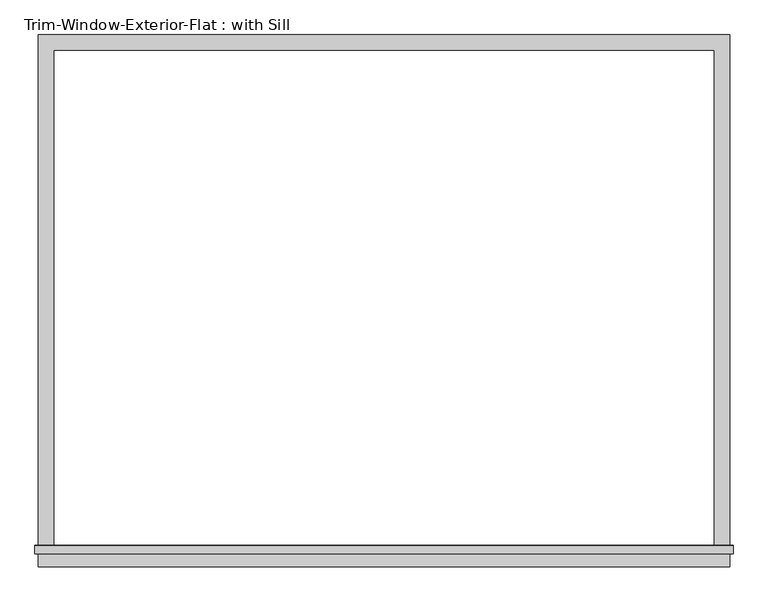
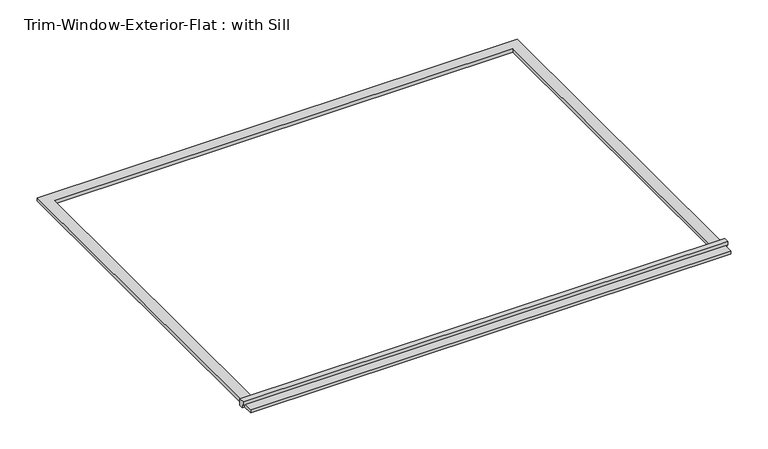
"""IFC4 building model written with IfcOpenShell, lengths in millimetres: proxy geometry, Trim-Window-Exterior-Flat : with Sill."""

from ifc_helpers import new_model, si_unit, frame, origin, origin_with_axes, place, context, project, spatial, polyline, outline, extrude, source, transform, mapped, element, save


def trim_window_exterior_flat_with_sill_359ed2ce(model_context):
    return source(origin(), model_context, "Body", "SweptSolid", [
        extrude(outline(polyline([(1276.35, -1850.9823709), (1276.35, -1908.1323709), (-1276.35, -1908.1323709), (-1276.35, -1850.9823709), (1276.35, -1850.9823709)])), origin_with_axes(), (0.0, 0.0, 1.0), 19.05),
        extrude(outline(polyline([(-1860.55, 38.1), (-1831.2580645, 38.1), (-1828.8, 19.05), (-1828.8, 0.0), (-1850.9823709, 0.0), (-1850.9823709, 19.05), (-1860.55, 19.05), (-1860.55, 38.1)])), frame((-1289.05, 0.0, 0.0), z_axis=(1.0, 0.0, 0.0), x_axis=(0.0, 1.0, 0.0)), (0.0, 0.0, 1.0), 2578.1),
        extrude(outline(polyline([(-1276.35, 57.15), (1276.35, 57.15), (1276.35, -1828.8), (1219.2, -1828.8), (1219.2, 0.0), (-1219.2, 0.0), (-1219.2, -1828.8), (-1276.35, -1828.8), (-1276.35, 57.15)])), origin_with_axes(), (0.0, 0.0, 1.0), 19.05),
    ])


if __name__ == "__main__":
    model = new_model("IFC4")
    model_context = context("Model", 3, world=origin())
    ifc_project = project(units=[si_unit("LENGTHUNIT", "METRE", prefix="MILLI")], contexts=[model_context])
    site = spatial("IfcSite", under=ifc_project)
    building = spatial("IfcBuilding", under=site)
    placement = place(None, origin())
    trim_window_exterior_flat_with_sill_shape = trim_window_exterior_flat_with_sill_359ed2ce(model_context)
    element("IfcBuildingElementProxy", 1, Name="Trim-Window-Exterior-Flat : with Sill", ObjectType="Trim-Window-Exterior-Flat : with Sill", at=placement, inside=building, context=model_context, shape_type="MappedRepresentation", body=[
        mapped(trim_window_exterior_flat_with_sill_shape, transform((0.0, 0.0, 0.0), x_axis=(1.0, 0.0, 0.0), y_axis=(0.0, 1.0, 0.0), z_axis=(0.0, 0.0, 1.0))),
    ])
    save(model, "model.ifc")

# Revit data of these elements
# Type "Trim-Window-Exterior-Flat : with Sill"
#   Trim Width = 0' - 2 1/4"
#   Trim Thickness_Picture Frame = 0' - 1 1/4"
#   Trim Thickness_with Sill = 0' - 0 3/4"
#   Sill Thickness = 0' - 1 1/4"
#   Opening Width [instance default] = 2' - 0"
#   Opening Height [instance default] = 3' - 0"
#   Default Elevation = 4' - 0"
#   Sill = yes
#   Picture Frame = no
#   Trim Material [instance default] = none
# Element 1 (IfcBuildingElementProxy, "Trim-Window-Exterior-Flat : with Sill")
#   Opening Width = 8' - 0"
#   Opening Height = 6' - 0"
#   Trim Material = Clad - White
#   Materials on its faces: "Clad - White"
# Materials
#   "Clad - White": class "Wood", colour RGB 242 242 238, transparency 0, Cost = 0
